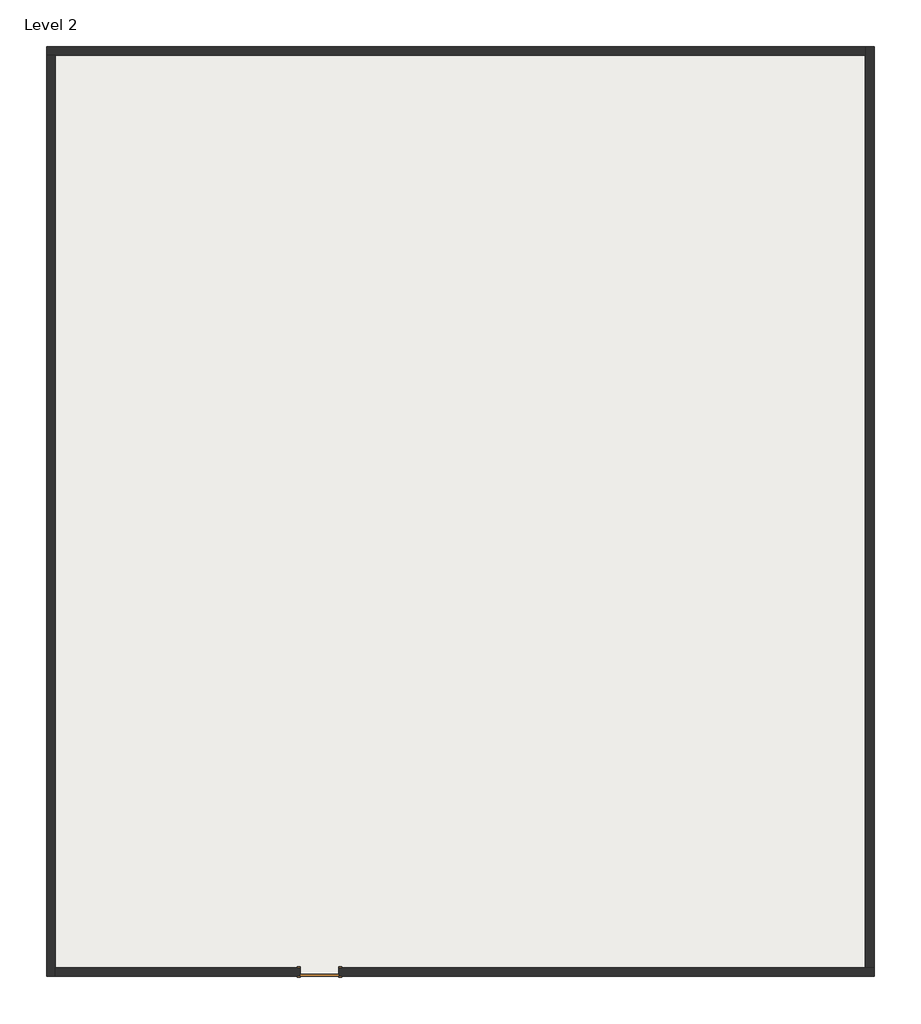
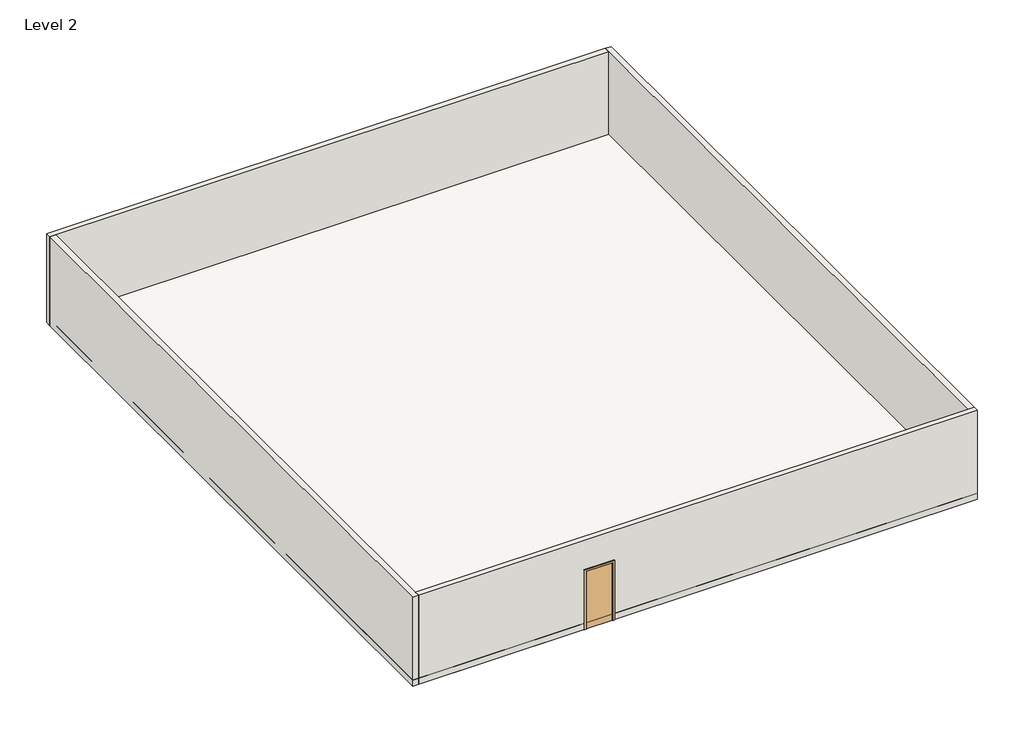
# One storey: 4 walls, 1 door, 1 roof.
"""IFC4 building model written with IfcOpenShell, lengths in millimetres."""

from ifc_helpers import new_model, si_unit, frame, origin, place, context, project, spatial, polyline, outline, extrude, faceted_brep, transform, mapped, element, save
from components import door_54dd4da4

model = new_model("IFC4")

# Units and contexts
model_context = context("Model", 3, world=origin())
ifc_project = project(units=[si_unit("LENGTHUNIT", "METRE", prefix="MILLI")], contexts=[model_context])

# Site, building, storey
site = spatial("IfcSite", under=ifc_project)
building = spatial("IfcBuilding", under=site)
storey = spatial("IfcBuildingStorey", under=building, Name="Level 2", Elevation=3048.0)

# Door
placement = place(None, origin())
door_shape = door_54dd4da4(model_context)
element("IfcDoor", 1, ObjectType="Single-Flush : 36\" x 84\"", at=placement, inside=storey, context=model_context, shape_type="MappedRepresentation", body=[
    mapped(door_shape, transform((-3456.7625896, -8539.5821053, 3048.0), x_axis=(-1.0, 0.0, 0.0), y_axis=(0.0, -1.0, 0.0), z_axis=(0.0, 0.0, 1.0))),
])

# Roof
element("IfcRoof", 2, ObjectType="Generic - 9\"", at=placement, inside=storey, context=model_context, shape_type="SweptSolid", body=[
    extrude(outline(polyline([(-9959.1625896, 13507.6178947), (9751.2374104, 13507.6178947), (9751.2374104, -8641.1821053), (-9959.1625896, -8641.1821053), (-9959.1625896, 13507.6178947)])), frame((0.0, 0.0, 3048.0), z_axis=(0.0, 0.0, 1.0), x_axis=(1.0, 0.0, 0.0)), (0.0, 0.0, 1.0), 228.6),
])

# Walls
element("IfcWall", 3, ObjectType="Generic - 8\"", at=placement, inside=storey, context=model_context, shape_type="Brep", body=[
    faceted_brep([(-9959.1625896, 13304.4178947, 3048.0), (-9755.9625896, 13304.4178947, 3048.0), (9548.0374104, 13304.4178947, 3048.0), (9548.0374104, 13304.4178947, 6324.6), (-9755.9625896, 13304.4178947, 6324.6), (-9959.1625896, 13304.4178947, 6324.6), (-9959.1625896, 13507.6178947, 3048.0), (-9959.1625896, 13507.6178947, 6324.6), (9548.0374104, 13507.6178947, 6324.6), (9548.0374104, 13507.6178947, 3048.0)], [[[0, 1, 2, 3, 4, 5]], [[6, 7, 8, 9]], [[2, 1, 0, 6, 9]], [[5, 4, 3, 8, 7]], [[0, 5, 7, 6]], [[3, 2, 9, 8]]]),
])
element("IfcWall", 4, ObjectType="Generic - 8\"", at=placement, inside=storey, context=model_context, shape_type="Brep", body=[
    faceted_brep([(-9755.9625896, -8641.1821053, 3048.0), (-9755.9625896, -8437.9821053, 3048.0), (-9755.9625896, 13304.4178947, 3048.0), (-9755.9625896, 13304.4178947, 6324.6), (-9755.9625896, -8437.9821053, 6324.6), (-9755.9625896, -8641.1821053, 6324.6), (-9959.1625896, -8641.1821053, 3048.0), (-9959.1625896, -8641.1821053, 6324.6), (-9959.1625896, 13304.4178947, 6324.6), (-9959.1625896, 13304.4178947, 3048.0)], [[[0, 1, 2, 3, 4, 5]], [[6, 7, 8, 9]], [[2, 1, 0, 6, 9]], [[5, 4, 3, 8, 7]], [[0, 5, 7, 6]], [[3, 2, 9, 8]]]),
])
element("IfcWall", 5, ObjectType="Generic - 8\"", at=placement, inside=storey, context=model_context, shape_type="Brep", body=[
    faceted_brep([(-3913.9625896, -8437.9821053, 5181.6), (-3913.9625896, -8437.9821053, 3048.0), (-9755.9625896, -8437.9821053, 3048.0), (-9755.9625896, -8437.9821053, 6324.6), (9548.0374104, -8437.9821053, 6324.6), (9751.2374104, -8437.9821053, 6324.6), (9751.2374104, -8437.9821053, 3048.0), (9548.0374104, -8437.9821053, 3048.0), (-2999.5625896, -8437.9821053, 3048.0), (-2999.5625896, -8437.9821053, 5181.6), (-9755.9625896, -8641.1821053, 3048.0), (-3913.9625896, -8641.1821053, 3048.0), (-3913.9625896, -8641.1821053, 5181.6), (-2999.5625896, -8641.1821053, 5181.6), (-2999.5625896, -8641.1821053, 3048.0), (9751.2374104, -8641.1821053, 3048.0), (9751.2374104, -8641.1821053, 6324.6), (-9755.9625896, -8641.1821053, 6324.6)], [[[0, 1, 2, 3, 4, 5, 6, 7, 8, 9]], [[10, 11, 12, 13, 14, 15, 16, 17]], [[2, 1, 11, 10]], [[8, 7, 6, 15, 14]], [[5, 4, 3, 17, 16]], [[6, 5, 16, 15]], [[3, 2, 10, 17]], [[12, 11, 1, 0]], [[13, 12, 0, 9]], [[14, 13, 9, 8]]]),
])
element("IfcWall", 6, ObjectType="Generic - 8\"", at=placement, inside=storey, context=model_context, shape_type="Brep", body=[
    faceted_brep([(9548.0374104, 13507.6178947, 3048.0), (9548.0374104, 13304.4178947, 3048.0), (9548.0374104, -8437.9821053, 3048.0), (9548.0374104, -8437.9821053, 6324.6), (9548.0374104, 13304.4178947, 6324.6), (9548.0374104, 13507.6178947, 6324.6), (9751.2374104, 13507.6178947, 3048.0), (9751.2374104, 13507.6178947, 6324.6), (9751.2374104, -8437.9821053, 6324.6), (9751.2374104, -8437.9821053, 3048.0)], [[[0, 1, 2, 3, 4, 5]], [[6, 7, 8, 9]], [[2, 1, 0, 6, 9]], [[5, 4, 3, 8, 7]], [[0, 5, 7, 6]], [[3, 2, 9, 8]]]),
])

save(model, "model.ifc")

# Revit data of these elements
# Type "Single-Flush : 36\" x 84\""
#   Type Mark = "1"
#   Construction Type Id = "MDOOR"
#   Assembly Code = "C1020"
#   Analytic Construction = "Metal"
#   Thickness = 0' - 2"
#   Heat Transfer Coefficient (U) = 0.651978 BTU/(h·ft²·°F)
#   Height = 7' - 0"
#   Trim Projection Ext = 0' - 1"
#   Trim Projection Int = 0' - 1"
#   Trim Width = 0' - 3"
#   Width = 3' - 0"
#   Define Thermal Properties by = 1
#   Door Material = Door - Panel
#   Frame Material = Door - Frame
#   Visual Light Transmittance = 0
#   Solar Heat Gain Coefficient = 0
#   Function = (empty or 0)
#   Wall Closure = (empty or 0)
# Type "Generic - 9\""
#   Assembly Code = "B1020"
#   Layers, outside or top first: 0' - 9" no material (function 1)
# Type "Generic - 8\""
#   Assembly Code = "B2010"
#   Layers, outside or top first: 0' - 8" no material (function 1)
# Element 1 (IfcDoor, "Single-Flush : 36\" x 84\"")
#   Phase Created = New Construction
#   Materials on its faces: "Door - Frame", "Door - Panel"
# Element 2 (IfcRoof, "Generic - 9\"")
#   built-in parameter 1001705 = 10.75 (stored number, unit not read)
#   built-in parameter 1001710 = 33615
#   Phase Created = New Construction
#   Materials on its faces: "Default Roof"
# Elements 3, 4, 5, 6 (IfcWall, "Generic - 8\"")
#   Top Offset = 0' - 0"
#   Base Offset = 0' - 0"
#   Unconnected Height = 10' - 9"
#   wall height = 10' - 9"
#   Phase Created = New Construction
#   Base Constraint = Level 2
#   Materials on its faces: "Default Wall"
# Materials
#   "Door - Panel": class "Wood", colour RGB 210 159 95, transparency 0
#   "Door - Frame": colour RGB 118 70 51, transparency 0
#   "Default Roof": colour RGB 88 101 114, transparency 0
#   "Default Wall": colour RGB 128 128 128, transparency 0
